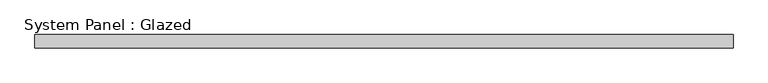
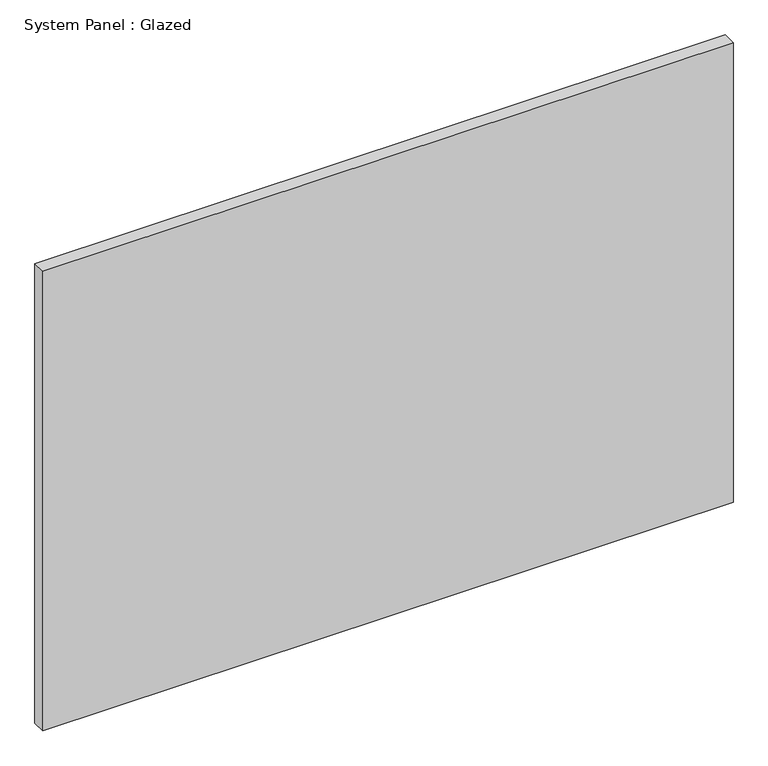
"""IFC4 building model written with IfcOpenShell, lengths in millimetres: plate geometry, System Panel : Glazed."""

from ifc_helpers import new_model, si_unit, origin, origin_with_axes, place, context, project, spatial, polyline, outline, extrude, source, transform, mapped, element, save


def system_panel_glazed_c1b4dd64(model_context):
    return source(origin(), model_context, "Body", "SweptSolid", [
        extrude(outline(polyline([(654.0499999, 19.05), (-654.0499999, 19.05), (-654.0499999, 44.45), (654.0499999, 44.45), (654.0499999, 19.05)])), origin_with_axes(), (0.0, 0.0, 1.0), 920.75),
    ])


if __name__ == "__main__":
    model = new_model("IFC4")
    model_context = context("Model", 3, world=origin())
    ifc_project = project(units=[si_unit("LENGTHUNIT", "METRE", prefix="MILLI")], contexts=[model_context])
    site = spatial("IfcSite", under=ifc_project)
    building = spatial("IfcBuilding", under=site)
    placement = place(None, origin())
    system_panel_glazed_shape = system_panel_glazed_c1b4dd64(model_context)
    element("IfcPlate", 1, ObjectType="System Panel : Glazed", at=placement, inside=building, context=model_context, shape_type="MappedRepresentation", body=[
        mapped(system_panel_glazed_shape, transform((0.0, 0.0, 0.0), x_axis=(1.0, 0.0, 0.0), y_axis=(0.0, 1.0, 0.0), z_axis=(0.0, 0.0, 1.0))),
    ])
    save(model, "model.ifc")

# Revit data of these elements
# Type "System Panel : Glazed"
#   Construction Type Id = "GSP4R"
#   Analytic Construction = "1/8 in Pilkington single glazing"
#   Visual Light Transmittance = 0.9
#   Solar Heat Gain Coefficient = 0.86
#   Heat Transfer Coefficient (U) = 1.18115 BTU/(h·ft²·°F)
#   Define Thermal Properties by = 1
# Element 1 (IfcPlate, "System Panel : Glazed")
#   Materials on its faces: "glass panel 223"
# Materials
#   "glass panel 223": class "Generic", colour RGB 120 120 120, transparency 0, Cost = 0
